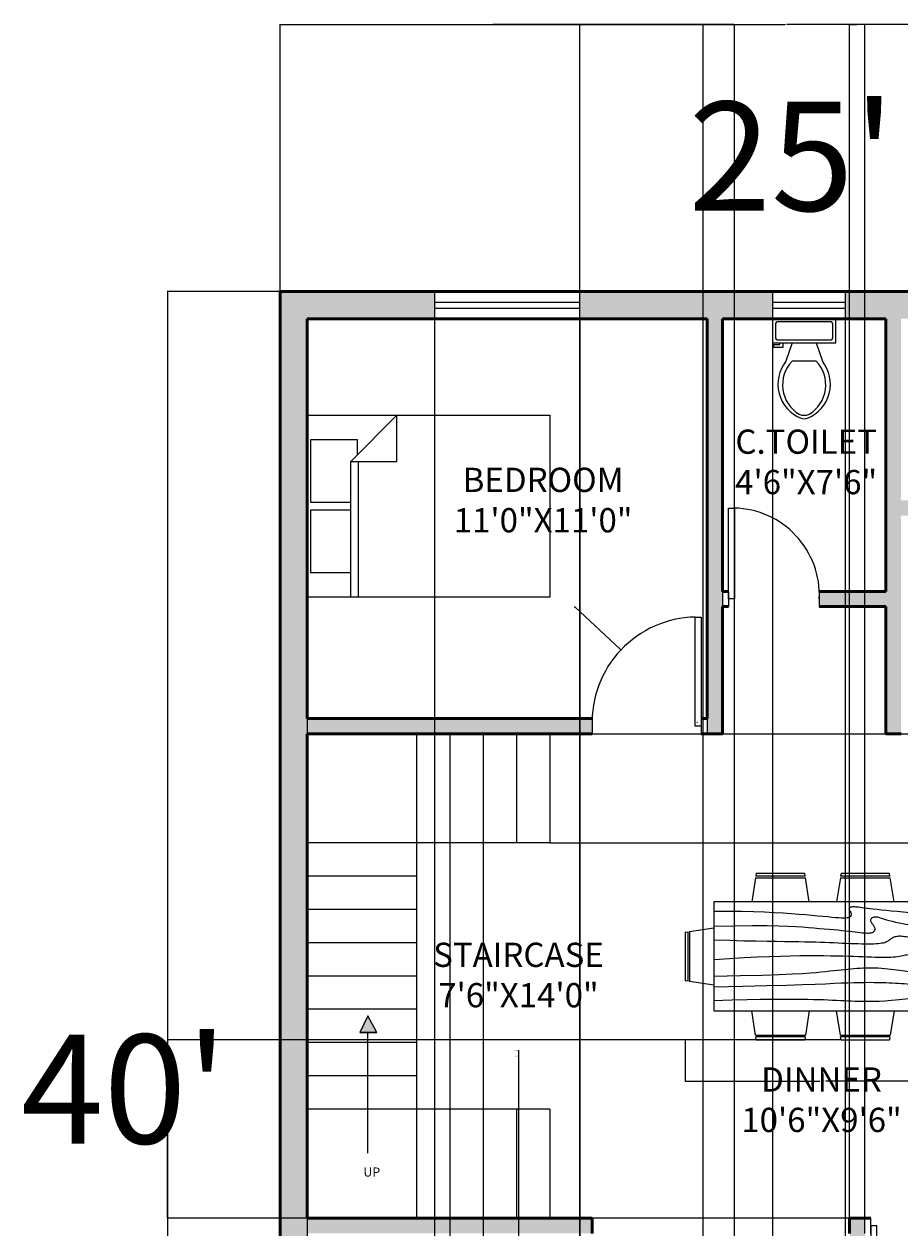
# Model space of a CAD drawing. Units: inches. Extents: x 76 to 532, y 199 to 998.
# Tile 3 of 4: x 76 to 365, y 601 to 998. Entities that reach past the tile are written whole.
import ezdxf

# ---------------------------------------------------------------- set-up
doc = ezdxf.new("R2010")
doc.units = ezdxf.units.IN
for name, color, linetype, lineweight in [('A-ANNO-DIMS', 2, 'Continuous', 18), ('A-ANNO-SYMB', 200, 'Continuous', 18), ('A-AREA-IDEN', 3, 'Continuous', 18), ('A-FLOR-FIXT', 8, 'Continuous', 18), ('A-FURN', 8, 'Continuous', 18), ('A-WALL', 7, 'Continuous', 50), ('A-WALL-PATT', 45, 'Continuous', 13), ('DIMENSION', 200, 'Continuous', 25), ('doors', 1, 'Continuous', 25), ('stairs', 6, 'Continuous', 25), ('windows', 140, 'Continuous', 18)]:
    doc.layers.add(name, color=color, linetype=linetype, lineweight=lineweight)
doc.styles.get("Standard").update_dxf_attribs({"font": 'arial.ttf'})
doc.dimstyles.get("Standard").update_dxf_attribs({"dimtxt": 0.18, "dimasz": 0.18, "dimexe": 0.18, "dimexo": 0.0625, "dimgap": 0.09, "dimtad": 0, "dimtih": 1, "dimtoh": 1, "dimdec": 4, "dimzin": 0, "dimdsep": 46, "dimtxsty": 'Standard', "dimcen": 0.09, "dimadec": 0, "dimazin": 0, "dimtfac": 1, "dimtdec": 4, "dimtofl": 0, "dimtmove": 0, "dimatfit": 3, "dimfxl": 1, "dimtolj": 1, "dimtzin": 0, "dimarcsym": 0})

# ---------------------------------------------------------------- blocks, each defined once
blk = doc.blocks.new('Bed - Queen')
for p, q in [((0, -80.00003), (0, 0)), ((0, 0), (59.99999, 0)), ((59.99999, 0), (59.99999, -80.00003)), ((7.99999, -1.2), (28.79998, -1.2)), ((7.99999, -14.4), (7.99999, -1.2)), ((28.79998, -1.2), (28.79998, -14.4)), ((31.19999, -1.2), (51.99999, -1.2)), ((31.19999, -14.4), (31.19999, -1.2)), ((51.99999, -1.2), (51.99999, -16.4)), ((0, -14.4), (44.8, -14.4)), ((59.99999, -29.6), (44.8, -14.4)), ((44.8, -14.4), (44.8, -29.6)), ((44.8, -16.8), (0, -16.8)), ((51.99999, -16.4), (46.79936, -16.4)), ((44.8, -29.6), (59.99999, -29.6)), ((59.99999, -80.00003), (0, -80.00003))]:
    blk.add_line(p, q)
blk = doc.blocks.new('Dining Set - 36 x 72 in.')
for p, q in [((-22.2343, 26.00059), (-23.4847, 17.99762)), ((-22.2304, 26), (-5.7608, 26)), ((-22, 27.5), (-22.1562, 26.50042)), ((-5.8416, 26.5), (-22.1534, 26.5)), ((-22, 27.5), (-6, 27.5)), ((-5.8437, 26.49966), (-6, 27.5)), ((-4.5152, 17.99762), (-5.7655, 25.99926)), ((5.7657, 26.00059), (4.5153, 17.99762)), ((5.7696, 26), (22.2392, 26)), ((6, 27.5), (5.8438, 26.50042)), ((22.1584, 26.5), (5.8466, 26.5)), ((6, 27.5), (22, 27.5)), ((22.1563, 26.49966), (22, 27.5)), ((23.4848, 17.99762), (22.2345, 25.99926)), ((36, 18), (-36, 18)), ((-36, 18), (-36, -18)), ((36, -18), (36, 18)), ((-45.5, 8), (-44.5004, 8.15617)), ((-45.5, 8), (-45.5, -8)), ((-44.5, -8.15843), (-44.5, 8.15338)), ((-44.0006, 8.23428), (-35.9976, 9.48474)), ((-44, 8.23041), (-44, -8.23915)), ((44.0006, 8.23428), (35.9976, 9.48474)), ((44, 8.23041), (44, -8.23915)), ((44.5, -8.15843), (44.5, 8.15338)), ((45.5, 8), (44.5005, 8.15617)), ((45.5, 8), (45.5, -8)), ((-44.4997, -8.15631), (-45.5, -8)), ((-35.9976, -9.48476), (-43.9993, -8.2345)), ((35.9976, -9.48476), (43.9993, -8.2345)), ((44.4997, -8.15631), (45.5, -8)), ((-36, -18), (36, -18)), ((-22.2343, -26.0006), (-23.4847, -17.99762)), ((-4.5152, -17.99762), (-5.7655, -25.99928)), ((5.7657, -26.0006), (4.5153, -17.99762)), ((23.4848, -17.99762), (22.2345, -25.99928)), ((-22.2304, -26), (-5.7608, -26)), ((-22, -27.5), (-22.1562, -26.50044)), ((-5.8416, -26.5), (-22.1534, -26.5)), ((-22, -27.5), (-6, -27.5)), ((-5.8437, -26.49967), (-6, -27.5)), ((5.7696, -26), (22.2392, -26)), ((6, -27.5), (5.8438, -26.50044)), ((22.1584, -26.5), (5.8466, -26.5)), ((6, -27.5), (22, -27.5)), ((22.1563, -26.49967), (22, -27.5))]:
    blk.add_line(p, q)
for points in [[(-36, 15), (-31.1772, 14.97754), (-26.8079, 14.91406), (-22.8538, 14.81543), (-19.276, 14.6875), (-16.0362, 14.53613), (-13.0957, 14.36718), (-10.4159, 14.18652), (-7.9583, 14), (-5.6904, 13.81315), (-3.6035, 13.63021), (-1.6954, 13.45508), (0.0365, 13.29166), (1.5945, 13.14388), (2.9811, 13.01562), (4.1988, 12.9108), (5.25, 12.83333), (6.1393, 12.78613), (6.8802, 12.76823), (7.4883, 12.77767), (7.9792, 12.8125), (8.3685, 12.87077), (8.6719, 12.95052), (8.9049, 13.0498), (9.0833, 13.16666), (9.2205, 13.29899), (9.3216, 13.44401), (9.3895, 13.59879), (9.4271, 13.76041), (9.4373, 13.92594), (9.4232, 14.09245), (9.3875, 14.257), (9.3333, 14.41666), (9.2638, 14.56917), (9.1836, 14.71484), (9.0975, 14.85465), (9.0104, 14.98958), (8.9272, 15.1206), (8.8529, 15.2487), (8.7922, 15.37483), (8.75, 15.5), (8.7305, 15.62467), (8.7344, 15.74739), (8.7617, 15.86621), (8.8125, 15.97916), (8.8867, 16.08431), (8.9844, 16.17968), (9.1055, 16.26334), (9.25, 16.33333), (9.4189, 16.38802), (9.6172, 16.42708), (9.8506, 16.45052), (10.125, 16.45833), (10.4463, 16.45052), (10.8203, 16.42708), (11.2529, 16.38802), (11.75, 16.33333), (12.3184, 16.26318), (12.9694, 16.17838), (13.7151, 16.07991), (14.5677, 15.96875), (15.5395, 15.84586), (16.6426, 15.71224), (17.8893, 15.56884), (19.2917, 15.41666), (20.859, 15.25667), (22.5879, 15.08984), (24.4721, 14.91715), (26.5052, 14.73958), (28.6809, 14.5581), (30.9929, 14.3737), (33.4347, 14.18733), (36, 14)], [(-36, 10), (-28.9766, 10.14274), (-23.1725, 10.20442), (-18.4241, 10.19775), (-14.5677, 10.13541), (-11.4399, 10.03011), (-8.877, 9.89453), (-6.7154, 9.74137), (-4.7917, 9.58333), (-2.9698, 9.43082), (-1.2246, 9.28515), (0.4415, 9.14534), (2.026, 9.01041), (3.5266, 8.87939), (4.9408, 8.7513), (6.266, 8.62516), (7.5, 8.5), (8.6411, 8.37549), (9.6914, 8.2539), (10.6538, 8.13818), (11.5312, 8.03125), (12.3267, 7.93603), (13.043, 7.85547), (13.6831, 7.79248), (14.25, 7.75), (14.7471, 7.7303), (15.1797, 7.73307), (15.5537, 7.75732), (15.875, 7.80208), (16.1494, 7.86637), (16.3828, 7.94922), (16.5811, 8.04964), (16.75, 8.16666), (16.8944, 8.29915), (17.0143, 8.44531), (17.1089, 8.60319), (17.1771, 8.77083), (17.218, 8.94629), (17.2305, 9.1276), (17.2137, 9.31282), (17.1667, 9.5), (17.0895, 9.6875), (16.987, 9.875), (16.8649, 10.0625), (16.7292, 10.25), (16.5856, 10.4375), (16.4401, 10.625), (16.2985, 10.8125), (16.1667, 11), (16.05, 11.18733), (15.9518, 11.3737), (15.8752, 11.5581), (15.8229, 11.73958), (15.798, 11.91715), (15.8034, 12.08984), (15.842, 12.25667), (15.9167, 12.41666), (16.0295, 12.56836), (16.1784, 12.70833), (16.3605, 12.83268), (16.5729, 12.9375), (16.8127, 13.01888), (17.0768, 13.07291), (17.3625, 13.0957), (17.6667, 13.08333), (17.9894, 13.03312), (18.3418, 12.94726), (18.7382, 12.82918), (19.1927, 12.68229), (19.7195, 12.51001), (20.3327, 12.31575), (21.0465, 12.10294), (21.875, 11.875), (22.8357, 11.63354), (23.959, 11.37304), (25.2786, 11.08618), (26.8282, 10.76562), (28.6414, 10.40405), (30.752, 9.99414), (33.1936, 9.52856), (36, 9)], [(-36, 5.5), (-30.7157, 5.3348), (-26.069, 5.20963), (-21.9946, 5.11767), (-18.4271, 5.05208), (-15.3009, 5.00602), (-12.5508, 4.97265), (-10.1112, 4.94515), (-7.9167, 4.91666), (-5.909, 4.88167), (-4.0586, 4.83984), (-2.3429, 4.79215), (-0.7396, 4.73958), (0.7739, 4.6831), (2.22, 4.6237), (3.6213, 4.56233), (5, 4.5), (6.373, 4.43782), (7.7344, 4.3776), (9.0723, 4.32129), (10.375, 4.27083), (11.6309, 4.22819), (12.8281, 4.19531), (13.9551, 4.17415), (15, 4.16666), (15.954, 4.17448), (16.819, 4.19791), (17.6001, 4.23698), (18.3021, 4.29166), (18.9299, 4.36198), (19.4883, 4.44791), (19.9823, 4.54948), (20.4167, 4.66666), (20.7969, 4.79899), (21.1302, 4.94401), (21.4245, 5.09879), (21.6875, 5.26041), (21.9271, 5.42594), (22.1511, 5.59245), (22.3672, 5.757), (22.5834, 5.91666), (22.8065, 6.06868), (23.0404, 6.21093), (23.2879, 6.34147), (23.5521, 6.45833), (23.8358, 6.55957), (24.142, 6.64323), (24.4735, 6.70735), (24.8334, 6.75), (25.2235, 6.76969), (25.642, 6.76692), (26.0858, 6.74267), (26.5521, 6.69791), (27.0379, 6.63362), (27.5404, 6.55078), (28.0565, 6.45036), (28.5834, 6.33333), (29.1242, 6.19987), (29.7071, 6.04687), (30.3661, 5.87044), (31.1354, 5.66666), (32.0493, 5.43164), (33.142, 5.16146), (34.4475, 4.85221), (36, 4.5)], [(-36, -1), (-30.7915, -0.6591), (-26.0195, -0.38216), (-21.6519, -0.16284), (-17.6563, 0.00521), (-14.0005, 0.12833), (-10.6523, 0.21289), (-7.5796, 0.26522), (-4.75, 0.29166), (-2.134, 0.29793), (0.2878, 0.28711), (2.5317, 0.26163), (4.6146, 0.22396), (6.5529, 0.17651), (8.3633, 0.12174), (10.0623, 0.06209), (11.6667, 0), (13.1899, -0.06201), (14.6341, -0.1211), (15.9982, -0.17432), (17.2813, -0.21875), (18.4823, -0.25147), (19.6003, -0.26953), (20.6343, -0.27002), (21.5834, -0.25), (22.4481, -0.20768), (23.2357, -0.14584), (23.9549, -0.06836), (24.6146, 0.02083), (25.2235, 0.11784), (25.7904, 0.21875), (26.3241, 0.31966), (26.8334, 0.41666), (27.3265, 0.50618), (27.8099, 0.58593), (28.2894, 0.65397), (28.7709, 0.70833), (29.2601, 0.74707), (29.763, 0.76823), (30.2855, 0.76985), (30.8334, 0.75), (31.4088, 0.70784), (31.9994, 0.64713), (32.589, 0.57275), (33.1615, 0.48958), (33.7008, 0.4025), (34.1908, 0.3164), (34.6153, 0.23616), (34.9584, 0.16666), (35.2099, 0.11165), (35.3848, 0.07031), (35.504, 0.04069), (35.5886, 0.02083), (35.6594, 0.00879), (35.7377, 0.0026), (35.8442, 0.00032), (36, 0)], [(-36, -6.5), (-27.1843, -6.31267), (-20.084, -6.1263), (-14.469, -5.9419), (-10.1094, -5.76042), (-6.7752, -5.58285), (-4.2363, -5.41016), (-2.2629, -5.24333), (-0.625, -5.08334), (0.8708, -4.93099), (2.2715, -4.78646), (3.5872, -4.64974), (4.8281, -4.52084), (6.0046, -4.39974), (7.127, -4.28646), (8.2053, -4.18099), (9.25, -4.08334), (10.2705, -3.99382), (11.2734, -3.91407), (12.2647, -3.84603), (13.25, -3.79167), (14.2354, -3.75293), (15.2266, -3.73177), (16.2295, -3.73015), (17.25, -3.75), (18.2912, -3.79248), (19.3451, -3.85547), (20.4009, -3.93604), (21.4479, -4.03125), (22.4754, -4.13819), (23.4727, -4.25391), (24.4289, -4.37549), (25.3334, -4.5), (26.1785, -4.62492), (26.9694, -4.74935), (27.7145, -4.87281), (28.4219, -4.99479), (29.1, -5.11483), (29.7572, -5.23242), (30.4016, -5.34709), (31.0417, -5.45834), (31.6837, -5.56437), (32.3262, -5.65821), (32.9658, -5.73153), (33.599, -5.77604), (34.2224, -5.78345), (34.8327, -5.74545), (35.4264, -5.65373), (36, -5.5)], [(-36, -10), (-26.4022, -9.81299), (-18.4675, -9.62891), (-11.9839, -9.45069), (-6.7396, -9.28125), (-2.5226, -9.12354), (0.8789, -8.98047), (3.6769, -8.85498), (6.0833, -8.75), (8.2767, -8.66765), (10.3021, -8.60677), (12.1712, -8.56543), (13.8958, -8.54167), (15.4876, -8.53353), (16.9583, -8.53907), (18.3197, -8.55632), (19.5834, -8.58334), (20.7616, -8.61841), (21.8685, -8.66081), (22.9188, -8.71004), (23.9271, -8.76563), (24.9081, -8.82707), (25.8763, -8.89388), (26.8465, -8.96558), (27.8334, -9.04167), (28.8474, -9.12118), (29.8828, -9.20117), (30.93, -9.27824), (31.9792, -9.34896), (33.0205, -9.40991), (34.0443, -9.45768), (35.0407, -9.48885), (36, -9.5)], [(-36, -14.5), (-30.0881, -14.33513), (-25.0332, -14.21224), (-20.7312, -14.12647), (-17.0781, -14.07292), (-13.97, -14.04671), (-11.3027, -14.04297), (-8.9724, -14.05681), (-6.875, -14.08334), (-4.9224, -14.11833), (-3.0905, -14.16016), (-1.3709, -14.20785), (0.2448, -14.26042), (1.7647, -14.3169), (3.1973, -14.3763), (4.5507, -14.43767), (5.8333, -14.5), (7.0554, -14.5621), (8.235, -14.62175), (9.3922, -14.67652), (10.5469, -14.72396), (11.7192, -14.76164), (12.929, -14.78711), (14.1965, -14.79794), (15.5417, -14.79167), (16.9933, -14.76424), (18.6152, -14.70508), (20.4804, -14.60197), (22.6615, -14.44271), (25.2312, -14.21509), (28.2624, -13.9069), (31.8277, -13.50594), (36, -13)]]:
    blk.add_lwpolyline(points)
blk = doc.blocks.new('*U10')
for p, q in [((9.5, -6), (9.5, -2)), ((-10, -8.5), (-8, -8.5)), ((-10, -9.5), (-10, -8.5)), ((-7, -9.5), (-10, -9.5)), ((-8, -8.5), (-8, -8)), ((-7, -8), (-7, -9.5)), ((-4, -8), (-6, -14)), ((4, -8), (6, -14)), ((4, -14), (-4, -14))]:
    blk.add_line(p, q)
blk.add_lwpolyline([(10.5, -8), (10.5, 0), (-10.5, 0), (-10.5, -8)], close=True)
for points in [[(-9.5, -2), (-9.5, -6)], [(8.5, -1), (-8.5, -1)], [(-8.5, -7), (8.5, -7)]]:
    blk.add_lwpolyline(points)
for centre, radius, start, end in [((-8.62, -1.88), 0.884, 81.8699, 188.1301), ((8.62, -1.88), 0.884, 351.8699, 98.1301), ((-8.62, -6.12), 0.884, 171.8699, 278.1301), ((8.62, -6.12), 0.884, 261.8699, 8.1301), ((3.52, -21.58), 12.17, 141.4691, 247.9714), ((4.2, -21.82), 11.33, 136.3677, 238.9468), ((-3.52, -21.58), 12.17, 292.0284, 38.5307), ((-4.2, -21.82), 11.33, 301.053, 43.6321), ((0, -27.88), 4, 245.7318, 294.2682), ((0, -29), 4, 254.8605, 285.1395)]:
    blk.add_arc(centre, radius, start, end)
blk = doc.blocks.new('glass')
at = {"layer": 'windows'}
for p, q in [((-12, 5.5), (-12, -3.5)), ((12, 5.5), (12, -3.5)), ((-12, 2), (12, 2)), ((-12, 0), (12, 0))]:
    blk.add_line(p, q, dxfattribs=at)
blk = doc.blocks.new('DOOR-SWING-30IN')
for p, q in [((0, 5), (0, 0)), ((2, 5), (2, 0)), ((32, 5), (32, 0))]:
    blk.add_line(p, q)
blk.add_lwpolyline([(2, 32.5), (4, 32.5), (4, 2.5), (2, 2.5)], close=True)
blk.add_arc((3.27, 3.75), 28.76, 357.5089, 88.5412)
blk = doc.blocks.new('WIN-48IN')
for p, q in [((0, 5.5), (48, 5.5)), ((0, 3.5), (48, 3.5))]:
    blk.add_line(p, q)
blk.add_lwpolyline([(0, 0), (48, 0), (48, 9), (0, 9)], close=True)
blk = doc.blocks.new('*D29')
at = {"layer": 'A-ANNO-DIMS', "color": 0, "lineweight": -2, "transparency": 16777216}
for p, q in [((294.53, 662.92), (294.53, 649.15)), ((385.53, 662.92), (385.53, 649.15)), ((294.71, 649.33), (339.08, 649.33)), ((385.35, 649.33), (340.98, 649.33))]:
    blk.add_line(p, q, dxfattribs=at)
at = {"layer": 'A-ANNO-DIMS', "color": 0, "transparency": 16777216}
for points in [[(294.71, 649.36), (294.71, 649.3), (294.53, 649.33)], [(385.35, 649.36), (385.35, 649.3), (385.53, 649.33)]]:
    blk.add_solid(points, dxfattribs=at)
at = {"layer": 'Defpoints', "color": 0, "transparency": 16777216}
for p in [(294.53, 662.98), (385.53, 662.98), (385.53, 649.33)]:
    blk.add_point(p, dxfattribs=at)
at = {"layer": 'A-ANNO-DIMS', "color": 0, "transparency": 16777216, "insert": (340.03, 649.33), "char_height": 0.18, "attachment_point": 5}
blk.add_mtext('\\A1;DINING SET 91', dxfattribs=at)
blk = doc.blocks.new('*D31')
at = {"layer": 'A-ANNO-DIMS', "color": 0, "lineweight": -2, "transparency": 16777216}
for p, q in [((160.86, 910.09), (160.86, 998.31)), ((161.04, 998.13), (327.57, 998.13)), ((494.68, 998.13), (328.15, 998.13)), ((494.86, 910.09), (494.86, 998.31))]:
    blk.add_line(p, q, dxfattribs=at)
at = {"layer": 'A-ANNO-DIMS', "color": 0, "transparency": 16777216}
for points in [[(161.04, 998.16), (161.04, 998.1), (160.86, 998.13)], [(494.68, 998.16), (494.68, 998.1), (494.86, 998.13)]]:
    blk.add_solid(points, dxfattribs=at)
at = {"layer": 'Defpoints', "color": 0, "transparency": 16777216}
for p in [(494.86, 998.13), (160.86, 910.03), (494.86, 910.03)]:
    blk.add_point(p, dxfattribs=at)
at = {"layer": 'A-ANNO-DIMS', "color": 0, "transparency": 16777216, "insert": (327.86, 998.13), "char_height": 0.18, "attachment_point": 5}
blk.add_mtext('\\A1;334', dxfattribs=at)
blk = doc.blocks.new('*D32')
at = {"layer": 'A-ANNO-DIMS', "color": 0, "lineweight": -2, "transparency": 16777216}
for p, q in [((160.79, 910.03), (123.58, 910.03)), ((123.76, 909.85), (123.76, 573.14)), ((123.76, 236.06), (123.76, 572.77)), ((320.39, 235.88), (123.58, 235.88))]:
    blk.add_line(p, q, dxfattribs=at)
at = {"layer": 'A-ANNO-DIMS', "color": 0, "transparency": 16777216}
for points in [[(123.73, 909.85), (123.79, 909.85), (123.76, 910.03)], [(123.73, 236.06), (123.79, 236.06), (123.76, 235.88)]]:
    blk.add_solid(points, dxfattribs=at)
at = {"layer": 'Defpoints', "color": 0, "transparency": 16777216}
for p in [(123.76, 910.03), (160.86, 910.03), (320.45, 235.88)]:
    blk.add_point(p, dxfattribs=at)
at = {"layer": 'A-ANNO-DIMS', "color": 0, "transparency": 16777216, "insert": (123.76, 572.95), "char_height": 0.18, "attachment_point": 5}
blk.add_mtext('\\A1;674.1', dxfattribs=at)
blk = doc.blocks.new('*D39')
at = {"layer": 'A-ANNO-DIMS', "color": 0, "lineweight": -2, "transparency": 16777216}
for p, q in [((169.86, 900.97), (169.86, 198.6)), ((211.86, 900.97), (211.86, 198.6)), ((170.04, 198.78), (190.64, 198.78)), ((211.68, 198.78), (191.08, 198.78))]:
    blk.add_line(p, q, dxfattribs=at)
at = {"layer": 'A-ANNO-DIMS', "color": 0, "transparency": 16777216}
for points in [[(170.04, 198.81), (170.04, 198.75), (169.86, 198.78)], [(211.68, 198.81), (211.68, 198.75), (211.86, 198.78)]]:
    blk.add_solid(points, dxfattribs=at)
at = {"layer": 'Defpoints', "color": 0, "transparency": 16777216}
for p in [(169.86, 901.03), (211.86, 901.03), (211.86, 198.78)]:
    blk.add_point(p, dxfattribs=at)
at = {"layer": 'A-ANNO-DIMS', "color": 0, "transparency": 16777216, "insert": (190.86, 198.78), "char_height": 0.18, "attachment_point": 5}
blk.add_mtext('\\A1;42', dxfattribs=at)
blk = doc.blocks.new('*D40')
at = {"layer": 'A-ANNO-DIMS', "color": 0, "lineweight": -2, "transparency": 16777216}
for p, q in [((259.86, 900.97), (259.86, 198.6)), ((323.36, 900.97), (323.36, 198.6)), ((260.04, 198.78), (291.28, 198.78)), ((323.18, 198.78), (291.93, 198.78))]:
    blk.add_line(p, q, dxfattribs=at)
at = {"layer": 'A-ANNO-DIMS', "color": 0, "transparency": 16777216}
for points in [[(260.04, 198.81), (260.04, 198.75), (259.86, 198.78)], [(323.18, 198.81), (323.18, 198.75), (323.36, 198.78)]]:
    blk.add_solid(points, dxfattribs=at)
at = {"layer": 'Defpoints', "color": 0, "transparency": 16777216}
for p in [(259.86, 901.03), (323.36, 901.03), (323.36, 198.78)]:
    blk.add_point(p, dxfattribs=at)
at = {"layer": 'A-ANNO-DIMS', "color": 0, "transparency": 16777216, "insert": (291.61, 198.78), "char_height": 0.18, "attachment_point": 5}
blk.add_mtext('\\A1;63.5', dxfattribs=at)
blk = doc.blocks.new('*D41')
at = {"layer": 'A-ANNO-DIMS', "color": 0, "lineweight": -2, "transparency": 16777216}
for p, q in [((347.36, 900.97), (347.36, 198.6)), ((401.86, 900.97), (401.86, 198.6)), ((347.54, 198.78), (374.28, 198.78)), ((401.68, 198.78), (374.93, 198.78))]:
    blk.add_line(p, q, dxfattribs=at)
at = {"layer": 'A-ANNO-DIMS', "color": 0, "transparency": 16777216}
for points in [[(347.54, 198.81), (347.54, 198.75), (347.36, 198.78)], [(401.68, 198.81), (401.68, 198.75), (401.86, 198.78)]]:
    blk.add_solid(points, dxfattribs=at)
at = {"layer": 'Defpoints', "color": 0, "transparency": 16777216}
for p in [(347.36, 901.03), (401.86, 901.03), (401.86, 198.78)]:
    blk.add_point(p, dxfattribs=at)
at = {"layer": 'A-ANNO-DIMS', "color": 0, "transparency": 16777216, "insert": (374.61, 198.78), "char_height": 0.18, "attachment_point": 5}
blk.add_mtext('\\A1;54.5', dxfattribs=at)
blk = doc.blocks.new('*D46')
at = {"layer": 'A-ANNO-DIMS', "color": 0, "lineweight": -2, "transparency": 16777216}
for p, q in [((249.92, 764.03), (532.14, 764.03)), ((531.96, 763.85), (531.96, 746.21)), ((531.96, 728.21), (531.96, 745.85)), ((249.92, 728.03), (532.14, 728.03))]:
    blk.add_line(p, q, dxfattribs=at)
at = {"layer": 'A-ANNO-DIMS', "color": 0, "transparency": 16777216}
for points in [[(531.93, 763.85), (531.99, 763.85), (531.96, 764.03)], [(531.93, 728.21), (531.99, 728.21), (531.96, 728.03)]]:
    blk.add_solid(points, dxfattribs=at)
at = {"layer": 'Defpoints', "color": 0, "transparency": 16777216}
for p in [(249.86, 764.03), (531.96, 764.03), (249.86, 728.03)]:
    blk.add_point(p, dxfattribs=at)
at = {"layer": 'A-ANNO-DIMS', "color": 0, "transparency": 16777216, "insert": (531.96, 746.03), "char_height": 0.18, "attachment_point": 5}
blk.add_mtext('\\A1;36', dxfattribs=at)
blk = doc.blocks.new('*D47')
at = {"layer": 'A-ANNO-DIMS', "color": 0, "lineweight": -2, "transparency": 16777216}
for p, q in [((216.86, 727.97), (216.86, 198.6)), ((227.86, 727.97), (227.86, 198.6)), ((217.04, 198.78), (222.16, 198.78)), ((227.68, 198.78), (222.55, 198.78))]:
    blk.add_line(p, q, dxfattribs=at)
at = {"layer": 'A-ANNO-DIMS', "color": 0, "transparency": 16777216}
for points in [[(217.04, 198.81), (217.04, 198.75), (216.86, 198.78)], [(227.68, 198.81), (227.68, 198.75), (227.86, 198.78)]]:
    blk.add_solid(points, dxfattribs=at)
at = {"layer": 'Defpoints', "color": 0, "transparency": 16777216}
for p in [(216.86, 728.03), (227.86, 728.03), (227.86, 198.78)]:
    blk.add_point(p, dxfattribs=at)
at = {"layer": 'A-ANNO-DIMS', "color": 0, "transparency": 16777216, "insert": (222.36, 198.78), "char_height": 0.18, "attachment_point": 5}
blk.add_mtext('\\A1;11', dxfattribs=at)
blk = doc.blocks.new('*D51')
at = {"layer": 'A-ANNO-DIMS', "color": 0, "lineweight": -2, "transparency": 16777216}
for p, q in [((259.86, 443.09), (259.86, 998.31)), ((260.04, 998.13), (285.16, 998.13)), ((310.68, 998.13), (285.56, 998.13)), ((310.86, 443.09), (310.86, 998.31))]:
    blk.add_line(p, q, dxfattribs=at)
at = {"layer": 'A-ANNO-DIMS', "color": 0, "transparency": 16777216}
for points in [[(260.04, 998.16), (260.04, 998.1), (259.86, 998.13)], [(310.68, 998.16), (310.68, 998.1), (310.86, 998.13)]]:
    blk.add_solid(points, dxfattribs=at)
at = {"layer": 'Defpoints', "color": 0, "transparency": 16777216}
for p in [(310.86, 998.13), (259.86, 443.03), (310.86, 443.03)]:
    blk.add_point(p, dxfattribs=at)
at = {"layer": 'A-ANNO-DIMS', "color": 0, "transparency": 16777216, "insert": (285.36, 998.13), "char_height": 0.18, "attachment_point": 5}
blk.add_mtext('\\A1;51', dxfattribs=at)
blk = doc.blocks.new('*D52')
at = {"layer": 'A-ANNO-DIMS', "color": 0, "lineweight": -2, "transparency": 16777216}
for p, q in [((160.86, 342.13), (160.86, 998.31)), ((161.04, 998.13), (230.22, 998.13)), ((300.31, 998.13), (231.13, 998.13)), ((300.49, 342.13), (300.49, 998.31))]:
    blk.add_line(p, q, dxfattribs=at)
at = {"layer": 'A-ANNO-DIMS', "color": 0, "transparency": 16777216}
for points in [[(161.04, 998.16), (161.04, 998.1), (160.86, 998.13)], [(300.31, 998.16), (300.31, 998.1), (300.49, 998.13)]]:
    blk.add_solid(points, dxfattribs=at)
at = {"layer": 'Defpoints', "color": 0, "transparency": 16777216}
for p in [(300.49, 998.13), (160.86, 342.07), (300.49, 342.07)]:
    blk.add_point(p, dxfattribs=at)
at = {"layer": 'A-ANNO-DIMS', "color": 0, "transparency": 16777216, "insert": (230.67, 998.13), "char_height": 0.18, "attachment_point": 5}
blk.add_mtext('\\A1;139.63', dxfattribs=at)
blk = doc.blocks.new('*D56')
at = {"layer": 'A-ANNO-DIMS', "color": 0, "lineweight": -2, "transparency": 16777216}
for p, q in [((348.86, 604.09), (348.86, 998.31)), ((349.04, 998.13), (351.21, 998.13)), ((353.68, 998.13), (351.51, 998.13)), ((353.86, 604.09), (353.86, 998.31))]:
    blk.add_line(p, q, dxfattribs=at)
at = {"layer": 'A-ANNO-DIMS', "color": 0, "transparency": 16777216}
for points in [[(349.04, 998.16), (349.04, 998.1), (348.86, 998.13)], [(353.68, 998.16), (353.68, 998.1), (353.86, 998.13)]]:
    blk.add_solid(points, dxfattribs=at)
at = {"layer": 'Defpoints', "color": 0, "transparency": 16777216}
for p in [(353.86, 998.13), (348.86, 604.03), (353.86, 604.03)]:
    blk.add_point(p, dxfattribs=at)
at = {"layer": 'A-ANNO-DIMS', "color": 0, "transparency": 16777216, "insert": (351.36, 998.13), "char_height": 0.18, "attachment_point": 5}
blk.add_mtext('\\A1;5', dxfattribs=at)
blk = doc.blocks.new('*D57')
at = {"layer": 'A-ANNO-DIMS', "color": 0, "lineweight": -2, "transparency": 16777216}
for p, q in [((345.97, 662.98), (123.58, 662.98)), ((123.76, 662.8), (123.76, 633.68)), ((123.76, 604.21), (123.76, 633.32)), ((348.79, 604.03), (123.58, 604.03))]:
    blk.add_line(p, q, dxfattribs=at)
at = {"layer": 'A-ANNO-DIMS', "color": 0, "transparency": 16777216}
for points in [[(123.73, 662.8), (123.79, 662.8), (123.76, 662.98)], [(123.73, 604.21), (123.79, 604.21), (123.76, 604.03)]]:
    blk.add_solid(points, dxfattribs=at)
at = {"layer": 'Defpoints', "color": 0, "transparency": 16777216}
for p in [(123.76, 662.98), (346.03, 662.98), (348.86, 604.03)]:
    blk.add_point(p, dxfattribs=at)
at = {"layer": 'A-ANNO-DIMS', "color": 0, "transparency": 16777216, "insert": (123.76, 633.5), "char_height": 0.18, "attachment_point": 5}
blk.add_mtext('\\A1;58.95', dxfattribs=at)
blk = doc.blocks.new('*D58')
at = {"layer": 'A-ANNO-DIMS', "color": 0, "lineweight": -2, "transparency": 16777216}
for p, q in [((257.98, 805.96), (258.16, 805.96)), ((258.16, 805.96), (273.19, 791.77)), ((298.5, 767.78), (298.68, 767.78)), ((298.59, 767.69), (298.59, 767.87))]:
    blk.add_line(p, q, dxfattribs=at)
at = {"layer": 'A-ANNO-DIMS', "color": 0, "transparency": 16777216}
blk.add_solid([(273.21, 791.79), (273.17, 791.74), (273.32, 791.64)], dxfattribs=at)
at = {"layer": 'Defpoints', "color": 0, "transparency": 16777216}
for p in [(273.32, 791.64), (298.59, 767.78)]:
    blk.add_point(p, dxfattribs=at)
at = {"layer": 'A-ANNO-DIMS', "color": 0, "transparency": 16777216, "insert": (257.31, 805.96), "char_height": 0.18, "attachment_point": 5}
blk.add_mtext('\\A1;2X R34.76', dxfattribs=at)
blk = doc.blocks.new('*D61')
at = {"layer": 'A-ANNO-DIMS', "color": 0, "lineweight": -2, "transparency": 16777216}
for p, q in [((239.33, 657.62), (239.51, 657.62)), ((239.51, 657.62), (239.51, 585.09)), ((239.42, 463.71), (239.6, 463.71)), ((239.51, 463.62), (239.51, 463.8))]:
    blk.add_line(p, q, dxfattribs=at)
at = {"layer": 'A-ANNO-DIMS', "color": 0, "transparency": 16777216}
blk.add_solid([(239.54, 585.09), (239.48, 585.09), (239.51, 584.91)], dxfattribs=at)
at = {"layer": 'Defpoints', "color": 0, "transparency": 16777216}
for p in [(239.51, 584.91), (239.51, 463.71)]:
    blk.add_point(p, dxfattribs=at)
at = {"layer": 'A-ANNO-DIMS', "color": 0, "transparency": 16777216, "insert": (238.85, 657.62), "char_height": 0.18, "attachment_point": 5}
blk.add_mtext('\\A1;R121.2', dxfattribs=at)
blk = doc.blocks.new('*D62')
at = {"layer": 'A-ANNO-DIMS', "color": 0, "lineweight": -2, "transparency": 16777216}
for p, q in [((239.33, 659.46), (239.51, 659.46)), ((239.51, 659.46), (239.51, 591.09)), ((239.42, 476.66), (239.6, 476.66)), ((239.51, 476.57), (239.51, 476.75))]:
    blk.add_line(p, q, dxfattribs=at)
at = {"layer": 'A-ANNO-DIMS', "color": 0, "transparency": 16777216}
blk.add_solid([(239.54, 591.09), (239.48, 591.09), (239.51, 590.91)], dxfattribs=at)
at = {"layer": 'Defpoints', "color": 0, "transparency": 16777216}
for p in [(239.51, 590.91), (239.51, 476.66)]:
    blk.add_point(p, dxfattribs=at)
at = {"layer": 'A-ANNO-DIMS', "color": 0, "transparency": 16777216, "insert": (238.78, 659.46), "char_height": 0.18, "attachment_point": 5}
blk.add_mtext('\\A1;R114.25', dxfattribs=at)

msp = doc.modelspace()

# ---------------------------------------------------------------- hatches: boundary and pattern name
at = {"layer": 'A-ANNO-SYMB'}
h = msp.add_hatch(color=256, dxfattribs=at)
h.dxf.hatch_style = 1
h.paths.add_polyline_path([(189.7806, 670.8873), (187.2357, 665.4259), (189.7806, 665.4259), (192.7912, 665.4259)])
at = {"layer": 'A-WALL-PATT'}
h = msp.add_hatch(color=256, dxfattribs=at)
h.dxf.hatch_style = 1
h.paths.add_polyline_path([(323.3571, 910.0275), (259.8571, 910.0275), (259.8571, 901.0275), (301.8571, 901.0275), (301.8571, 769.0275), (301.8571, 764.0275), (306.8571, 764.0275), (306.8571, 806.0275), (306.8571, 811.0275), (306.8571, 901.0275), (323.3571, 901.0275)])
h.paths.add_polyline_path([(211.8571, 910.0275), (160.8571, 910.0275), (160.8571, 539.5719), (169.8571, 539.5719), (169.8571, 599.0275), (263.8571, 599.0275), (263.8571, 604.0275), (169.8571, 604.0275), (169.8571, 764.0275), (263.8571, 764.0275), (263.8571, 766.5275, -0.0179874), (263.8571, 769.0275), (169.8571, 769.0275), (169.8571, 901.0275), (211.8571, 901.0275)])
h.paths.add_polyline_path([(401.8571, 910.0275), (347.3571, 910.0275), (347.3571, 901.0275), (360.8571, 901.0275), (360.8571, 811.0275), (338.8571, 811.0275, -0.02174236), (338.8571, 808.5275), (338.8571, 806.0275), (360.8571, 806.0275), (360.8571, 764.0275), (365.8571, 764.0275), (365.8571, 836.0275), (397.3621, 836.0275), (397.3621, 841.0275), (365.8571, 841.0275), (365.8571, 901.0275), (401.8571, 901.0275)])
h.paths.add_polyline_path([(169.8571, 479.5719), (160.8571, 479.5719), (160.8571, 434.0275), (211.8571, 434.0275), (211.8571, 443.0275), (169.8571, 443.0275)])
h.paths.add_polyline_path([(310.8571, 443.0275), (259.8571, 443.0275), (259.8571, 434.0275), (310.8571, 434.0275), (310.8571, 438.5275, -0.03336892)])
h.paths.add_polyline_path([(353.8571, 599.0275), (353.8571, 604.0275), (348.8571, 604.0275), (348.8571, 599.0275), (348.8571, 443.0275), (348.8571, 434.0275), (396.8571, 434.0275), (396.8571, 443.0275), (353.8571, 443.0275)])
h.paths.add_polyline_path([(494.8571, 619.5776), (485.8571, 619.5776), (485.8571, 604.0275), (427.8571, 604.0275, -0.02174236), (427.8571, 601.5275), (427.8571, 599.0275), (485.8571, 599.0275), (485.8571, 443.0275), (444.8571, 443.0275), (444.8571, 434.0275), (494.8571, 434.0275)])
h.paths.add_polyline_path([(494.8571, 673.4729), (485.8571, 673.4729), (485.8571, 663.0275), (431.8571, 663.0275), (431.8571, 711.0275), (431.8571, 716.0275), (426.8571, 716.0275), (426.8571, 663.0275), (390.8571, 663.0275), (390.8571, 604.0275), (385.8571, 604.0275), (385.8571, 601.5275, -0.02174236), (385.8571, 599.0275), (395.8571, 599.0275), (395.8571, 604.0275), (395.8571, 658.0275), (430.3571, 658.0275), (430.3571, 659.0275), (451.3571, 659.0275), (451.3571, 658.0275), (485.8571, 658.0275), (485.8571, 643.5776), (494.8571, 643.5776)])
h.paths.add_polyline_path([(494.8571, 752.0275), (485.8571, 752.0275), (485.8571, 716.0275), (463.8571, 716.0275), (463.8571, 713.5275, -0.02174236), (463.8571, 711.0275), (485.8571, 711.0275), (485.8571, 697.4729), (494.8571, 697.4729)])
h.paths.add_polyline_path([(494.8571, 910.0275), (449.8571, 910.0275), (449.8571, 901.0275), (485.8571, 901.0275), (485.8571, 841.0275), (429.3621, 841.0275, -0.02174236), (429.3621, 838.5275), (429.3621, 836.0275), (485.8571, 836.0275), (485.8571, 800.0275), (494.8571, 800.0275)])

# ---------------------------------------------------------------- linework, layer by layer
at = {"layer": 'A-ANNO-SYMB'}
for p, q in [((189.7806, 670.8873), (187.2357, 665.4259)), ((192.7912, 665.4259), (189.7806, 670.8873)), ((192.7912, 665.4259), (187.2357, 665.4259)), ((187.2357, 665.4259), (189.7806, 665.4259)), ((189.7806, 662.0275), (189.7806, 665.4259)), ((189.7806, 665.4259), (192.7912, 665.4259)), ((189.7806, 625.5589), (189.7806, 662.0275))]:
    msp.add_line(p, q, dxfattribs=at)
at = {"layer": 'A-WALL'}
for p, q in [((494.8571, 910.0275), (160.8571, 910.0275)), ((160.8571, 910.0275), (160.8571, 434.0275)), ((169.8571, 901.0275), (169.8571, 769.0275)), ((301.8571, 901.0275), (169.8571, 901.0275)), ((301.8571, 901.0275), (301.8571, 769.0275)), ((306.8571, 901.0275), (306.8571, 811.0275)), ((360.8571, 901.0275), (306.8571, 901.0275)), ((360.8571, 901.0275), (360.8571, 811.0275)), ((308.8571, 811.0275), (306.8571, 811.0275)), ((360.8571, 811.0275), (338.8571, 811.0275)), ((306.8571, 806.0275), (306.8571, 764.0275)), ((308.8571, 806.0275), (306.8571, 806.0275)), ((360.8571, 806.0275), (338.8571, 806.0275)), ((360.8571, 806.0275), (360.8571, 764.0275)), ((263.8571, 769.0275), (169.8571, 769.0275)), ((301.8571, 769.0275), (299.8571, 769.0275)), ((169.8571, 764.0275), (169.8571, 604.0275)), ((263.8571, 764.0275), (169.8571, 764.0275)), ((306.8571, 764.0275), (299.8571, 764.0275)), ((365.8571, 764.0275), (360.8571, 764.0275)), ((263.8571, 604.0275), (169.8571, 604.0275)), ((263.8571, 604.0275), (263.8571, 599.0275)), ((348.8571, 599.0275), (348.8571, 604.0275)), ((355.8571, 604.0275), (348.8571, 604.0275))]:
    msp.add_line(p, q, dxfattribs=at)
at = {"layer": 'doors'}
for p, q in [((263.8571, 769.0275), (263.8571, 764.0275)), ((299.8571, 769.0275), (299.8571, 764.0275)), ((301.8571, 769.0275), (301.8571, 764.0275))]:
    msp.add_line(p, q, dxfattribs=at)
msp.add_lwpolyline([(297.8571, 802.5275), (299.8571, 802.5275), (299.8571, 766.5275), (297.8571, 766.5275)], close=True, dxfattribs=at)
msp.add_arc((298.5923, 767.7775), 34.7578, 91.212172, 182.060982, dxfattribs=at)
at = {"layer": 'stairs'}
for p, q in [((205.8571, 764.0275), (205.8571, 604.0275)), ((216.8571, 764.0275), (216.8571, 728.0275)), ((227.8571, 764.0275), (227.8571, 728.0275)), ((238.8571, 764.0275), (238.8571, 728.0275)), ((249.8571, 764.0275), (249.8571, 728.0275)), ((249.8571, 728.0275), (169.8571, 728.0275)), ((205.8571, 717.0275), (169.8571, 717.0275)), ((205.8571, 706.0275), (169.8571, 706.0275)), ((205.8571, 695.0275), (169.8571, 695.0275)), ((205.8571, 684.0275), (169.8571, 684.0275)), ((205.8571, 673.0275), (169.8571, 673.0275)), ((205.8571, 662.0275), (169.8571, 662.0275)), ((205.8571, 651.0275), (169.8571, 651.0275)), ((249.8571, 640.0275), (169.8571, 640.0275)), ((216.8571, 640.0275), (216.8571, 604.0275)), ((227.8571, 640.0275), (227.8571, 604.0275)), ((238.8571, 640.0275), (238.8571, 604.0275)), ((249.8571, 640.0275), (249.8571, 604.0275))]:
    msp.add_line(p, q, dxfattribs=at)

# ---------------------------------------------------------------- block references
at = {"layer": 'A-FLOR-FIXT'}
msp.add_blockref('*U10', (333.8571, 901.0275), dxfattribs=at)
at = {"layer": 'A-FURN', "rotation": 90}
msp.add_blockref('Bed - Queen', (169.8571, 809.1366), dxfattribs=at)
at = {"layer": 'A-FURN'}
msp.add_blockref('Dining Set - 36 x 72 in.', (340.0288, 690.4778), dxfattribs=at)
at = {"layer": 'doors'}
msp.add_blockref('DOOR-SWING-30IN', (306.8571, 806.0275), dxfattribs=at)
at = {"layer": 'doors', "extrusion": (0, 0, -1), "zscale": -1, "rotation": 180}
msp.add_blockref('DOOR-SWING-30IN', (-353.8571, 604.0275), dxfattribs=at)
at = {"layer": 'windows'}
for name, p in [('WIN-48IN', (211.8571, 901.0275)), ('glass', (335.3571, 904.5275))]:
    msp.add_blockref(name, p, dxfattribs=at)

# ---------------------------------------------------------------- texts
at = {"layer": 'A-ANNO-SYMB', "insert": (188.3715, 620.8154), "char_height": 3, "attachment_point": 1}
msp.add_mtext_dynamic_manual_height_columns('UP', width=15.333903, gutter_width=12.5, heights=[0], dxfattribs=at)
at = {"layer": 'A-AREA-IDEN', "char_height": 8, "attachment_point": 1}
for s, insert in [('\\pxqc;C.TOILET\\P4\'6"X7\'6"', (294.2201, 864.4372)), ('\\pxqc;BEDROOM\\P11\'0"X11\'0"', (207.3882, 851.8359)), ('\\pxqc;STAIRCASE\\P7\'6"X14\'0"', (199.2461, 695.0275)), ('\\pxqc;DINNER\\P10\'6"X9\'6"', (299.2814, 653.8568))]:
    msp.add_mtext_dynamic_manual_height_columns(s, width=80.600486, gutter_width=12.5, heights=[0], dxfattribs=dict(at, insert=insert))
at = {"layer": 'DIMENSION', "char_height": 36, "attachment_point": 1}
for s, insert in [("25'", (295.6802, 972.6595)), ("40'", (75.3844, 664.7097))]:
    msp.add_mtext_dynamic_manual_height_columns(s, width=108.883863, gutter_width=12.5, heights=[0], dxfattribs=dict(at, insert=insert))

# ---------------------------------------------------------------- dimensions: what is measured, and where the dimension line sits
at = {"layer": 'A-ANNO-DIMS'}
for base, p1, p2, override, picture, middle in [((494.8571, 998.1275), (160.8571, 910.0275), (494.8571, 910.0275), {"dimdec": 0, "dimlfac": 1, "dimrnd": 0, "dimzin": 0, "dimdsep": 46, "dimlunit": 2}, '*D31', (327.8571, 998.1275)), ((300.4881, 998.1275), (160.8571, 342.0718), (300.4881, 342.0718), {"dimdec": 2, "dimlfac": 1, "dimrnd": 0, "dimzin": 0, "dimdsep": 46, "dimlunit": 2}, '*D52', (230.6726, 998.1275)), ((310.8571, 998.1275), (259.8571, 443.0275), (310.8571, 443.0275), {"dimdec": 0, "dimlfac": 1, "dimrnd": 0, "dimzin": 0, "dimdsep": 46, "dimlunit": 2}, '*D51', (285.3571, 998.1275)), ((353.8571, 998.1275), (348.8571, 604.0275), (353.8571, 604.0275), {"dimdec": 0, "dimlfac": 1, "dimrnd": 0, "dimzin": 0, "dimdsep": 46, "dimlunit": 2}, '*D56', (351.3571, 998.1275)), ((211.8571, 198.779), (169.8571, 901.0275), (211.8571, 901.0275), {"dimdec": 0, "dimlfac": 1, "dimrnd": 0, "dimzin": 0, "dimdsep": 46, "dimlunit": 2}, '*D39', (190.8571, 198.779)), ((323.3571, 198.779), (259.8571, 901.0275), (323.3571, 901.0275), {"dimdec": 1, "dimlfac": 1, "dimrnd": 0, "dimzin": 0, "dimdsep": 46, "dimlunit": 2}, '*D40', (291.6071, 198.779)), ((401.8571, 198.779), (347.3571, 901.0275), (401.8571, 901.0275), {"dimdec": 1, "dimlfac": 1, "dimrnd": 0, "dimzin": 0, "dimdsep": 46, "dimlunit": 2}, '*D41', (374.6071, 198.779)), ((227.8571, 198.779), (216.8571, 728.0275), (227.8571, 728.0275), {"dimdec": 0, "dimlfac": 1, "dimrnd": 0, "dimzin": 0, "dimdsep": 46, "dimlunit": 2}, '*D47', (222.3571, 198.779))]:
    dim = msp.add_linear_dim(base=base, p1=p1, p2=p2, dimstyle='Standard', override=override, dxfattribs=at)
    dim.commit()
    dim.dimension.update_dxf_attribs({"geometry": picture, "text_midpoint": middle})
for base, p1, p2, override, picture, middle in [((123.7571, 910.0275), (320.4491, 235.879), (160.8571, 910.0275), {"dimdec": 1, "dimlfac": 1, "dimrnd": 0, "dimzin": 0, "dimdsep": 46, "dimlunit": 2}, '*D32', (123.7571, 572.9533)), ((531.9571, 764.0275), (249.8571, 728.0275), (249.8571, 764.0275), {"dimdec": 0, "dimlfac": 1, "dimrnd": 0, "dimzin": 0, "dimdsep": 46, "dimlunit": 2}, '*D46', (531.9571, 746.0275)), ((123.7571, 662.9778), (348.8571, 604.0275), (346.0288, 662.9778), {"dimdec": 2, "dimlfac": 1, "dimrnd": 0, "dimzin": 0, "dimdsep": 46, "dimlunit": 2}, '*D57', (123.7571, 633.5026))]:
    dim = msp.add_linear_dim(base=base, p1=p1, p2=p2, angle=90, dimstyle='Standard', override=override, dxfattribs=at)
    dim.commit()
    dim.dimension.update_dxf_attribs({"geometry": picture, "text_midpoint": middle})
dim = msp.add_radius_dim(center=(298.5923, 767.7775), mpoint=(273.323, 791.643), text='2X <>', dimstyle='Standard', override={"dimdec": 2, "dimlfac": 1, "dimrnd": 0, "dimzin": 0, "dimdsep": 46, "dimlunit": 2}, dxfattribs=at)
dim.commit()
dim.dimension.update_dxf_attribs({"geometry": '*D58', "text_midpoint": (257.3067, 805.9623), "dimtype": 164})
dim = msp.add_linear_dim(base=(385.5288, 649.3278), p1=(294.5288, 662.9778), p2=(385.5288, 662.9778), text='DINING SET <>', dimstyle='Standard', override={"dimdec": 0, "dimlfac": 1, "dimrnd": 0, "dimzin": 0, "dimdsep": 46, "dimlunit": 2}, dxfattribs=at)
dim.commit()
dim.dimension.update_dxf_attribs({"geometry": '*D29', "text_midpoint": (340.0288, 649.3278)})
for center, mpoint, override, picture, middle in [((239.5062, 476.6561), (239.506, 590.9061), {"dimdec": 2, "dimlfac": 1, "dimrnd": 0, "dimzin": 0, "dimdsep": 46, "dimlunit": 2}, '*D62', (238.7755, 659.4561)), ((239.5062, 463.7093), (239.506, 584.9061), {"dimdec": 1, "dimlfac": 1, "dimrnd": 0, "dimzin": 0, "dimdsep": 46, "dimlunit": 2}, '*D61', (238.847, 657.6242))]:
    dim = msp.add_radius_dim(center=center, mpoint=mpoint, dimstyle='Standard', override=override, dxfattribs=at)
    dim.commit()
    dim.dimension.update_dxf_attribs({"geometry": picture, "text_midpoint": middle, "dimtype": 164})

doc.saveas('drawing.dxf')
